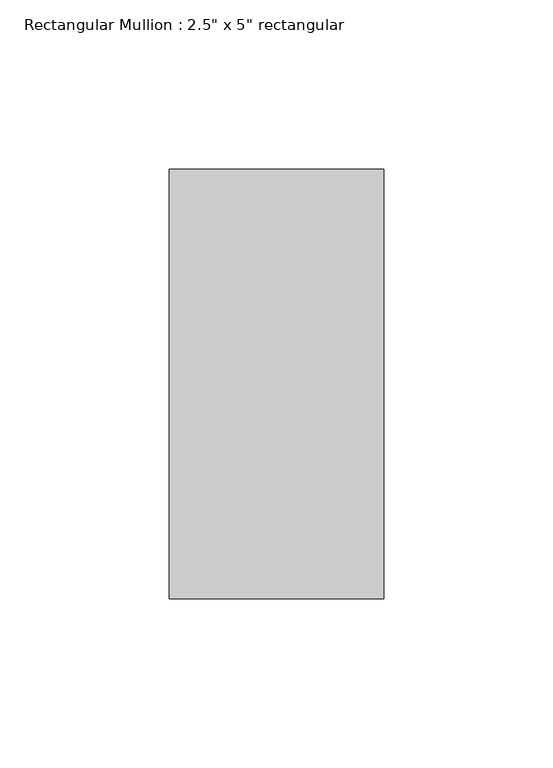
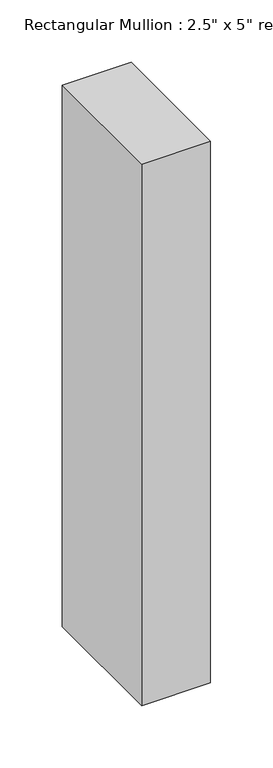
"""IFC4 building model written with IfcOpenShell, lengths in millimetres: member geometry."""

from ifc_helpers import new_model, si_unit, frame, origin, place, context, project, spatial, polyline, outline, extrude, source, transform, mapped, element, save


def member_f209f73c(model_context):
    return source(origin(), model_context, "Body", "SweptSolid", [
        extrude(outline(polyline([(31.75, 63.5), (31.75, -63.5), (-31.75, -63.5), (-31.75, 63.5), (31.75, 63.5)])), frame((0.0, 0.0, -529.1666667), z_axis=(0.0, 0.0, 1.0), x_axis=(1.0, 0.0, 0.0)), (0.0, 0.0, 1.0), 529.1666667),
    ])


if __name__ == "__main__":
    model = new_model("IFC4")
    model_context = context("Model", 3, world=origin())
    ifc_project = project(units=[si_unit("LENGTHUNIT", "METRE", prefix="MILLI")], contexts=[model_context])
    site = spatial("IfcSite", under=ifc_project)
    building = spatial("IfcBuilding", under=site)
    placement = place(None, origin())
    member_shape = member_f209f73c(model_context)
    element("IfcMember", 1, ObjectType="Rectangular Mullion : 2.5\" x 5\" rectangular", at=placement, inside=building, context=model_context, shape_type="MappedRepresentation", body=[
        mapped(member_shape, transform((0.0, 0.0, 0.0), x_axis=(1.0, 0.0, 0.0), y_axis=(0.0, 1.0, 0.0), z_axis=(0.0, 0.0, 1.0))),
    ])
    save(model, "model.ifc")

# Revit data of these elements
# Type "Rectangular Mullion : 2.5\" x 5\" rectangular"
#   built-in parameter 1007304 = 0.416667 (stored number, unit not read)
#   built-in parameter 1007301 = 0.104167 (stored number, unit not read)
#   built-in parameter 1007300 = 0.104167 (stored number, unit not read)
# Element 1 (IfcMember, "Rectangular Mullion : 2.5\" x 5\" rectangular")
#   Materials on its faces: "Aluminum"
# Materials
#   "Aluminum": class "Metal", colour RGB 247 247 247, transparency 0, Description = "Aluminum 6061", Cost = 0
